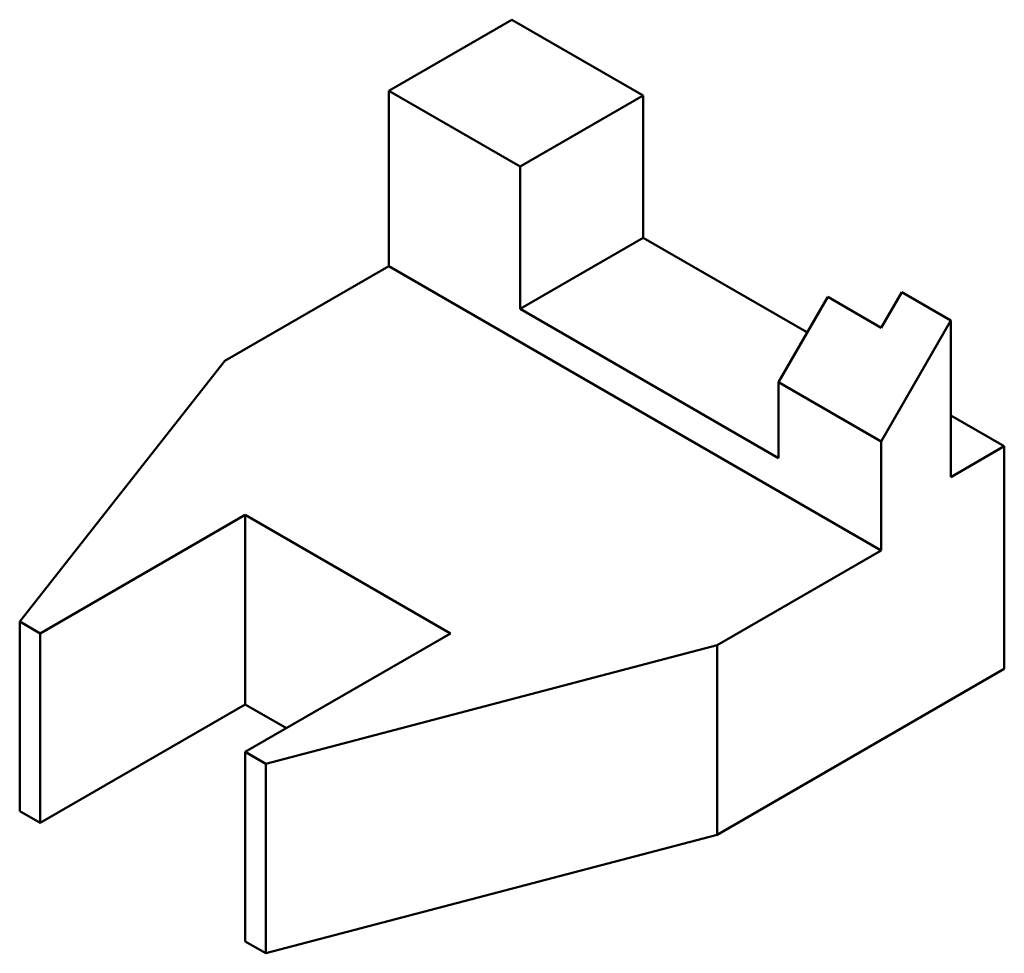
# Model space of a CAD drawing. Units: inches. Extents: x 17467 to 446717, y 8017 to 206428.
# Tile 2 of 2: x 444078 to 446717, y 203926 to 206428. Entities that reach past the tile are written whole.
import ezdxf

# ---------------------------------------------------------------- set-up
doc = ezdxf.new("R2010")
doc.units = ezdxf.units.IN
doc.layers.add('M-OUTL', color=7, linetype='Continuous', lineweight=50)

msp = doc.modelspace()

# ---------------------------------------------------------------- linework, layer by layer
at = {"layer": 'M-OUTL'}
for p, q in [((445067.6, 206237.5), (445397.5, 206428)), ((445749.5, 206224.8), (445397.5, 206428)), ((445067.6, 206237.5), (445067.6, 205767.6)), ((445419.5, 206034.3), (445067.6, 206237.5)), ((445419.5, 206034.3), (445749.5, 206224.8)), ((445749.5, 205843.8), (445749.5, 206224.8)), ((445419.5, 205653.3), (445419.5, 206034.3)), ((445419.5, 205653.3), (445749.5, 205843.8)), ((446189.4, 205589.8), (445749.5, 205843.8)), ((445067.6, 205767.6), (444627.6, 205513.6)), ((446387.4, 205005.6), (445067.6, 205767.6)), ((446244.4, 205685.1), (446112.4, 205456.5)), ((446387.4, 205602.5), (446244.4, 205685.1)), ((446442.4, 205697.8), (446387.4, 205602.5)), ((446574.4, 205621.6), (446442.4, 205697.8)), ((446112.4, 205253.3), (445419.5, 205653.3)), ((446574.4, 205621.6), (446387.4, 205297.7)), ((446574.4, 205202.5), (446574.4, 205621.6)), ((444627.6, 205513.6), (444077.7, 204815.1)), ((446112.4, 205456.5), (446112.4, 205253.3)), ((446387.4, 205297.7), (446112.4, 205456.5)), ((446717.4, 205285), (446574.4, 205367.6)), ((446387.4, 205297.7), (446387.4, 205005.6)), ((446574.4, 205202.5), (446717.4, 205285)), ((446717.4, 204688.1), (446717.4, 205285)), ((444132.7, 204783.4), (444682.6, 205100.9)), ((445232.6, 204783.4), (444682.6, 205100.9)), ((444682.6, 204592.9), (444682.6, 205100.9)), ((445947.5, 204751.6), (446387.4, 205005.6)), ((444077.7, 204815.1), (444132.7, 204783.4)), ((444077.7, 204307.1), (444077.7, 204815.1)), ((444132.7, 204275.4), (444132.7, 204783.4)), ((444682.6, 204465.9), (445232.6, 204783.4)), ((444737.6, 204434.1), (445947.5, 204751.6)), ((445947.5, 204243.6), (445947.5, 204751.6)), ((445947.5, 204243.6), (446717.4, 204688.1)), ((444132.7, 204275.4), (444682.6, 204592.9)), ((444792.6, 204529.4), (444682.6, 204592.9)), ((444682.6, 204465.9), (444737.6, 204434.1)), ((444682.6, 203957.9), (444682.6, 204465.9)), ((444737.6, 203926.1), (444737.6, 204434.1)), ((444077.7, 204307.1), (444132.7, 204275.4)), ((444737.6, 203926.1), (445947.5, 204243.6)), ((444682.6, 203957.9), (444737.6, 203926.1))]:
    msp.add_line(p, q, dxfattribs=at)

doc.saveas('drawing.dxf')
